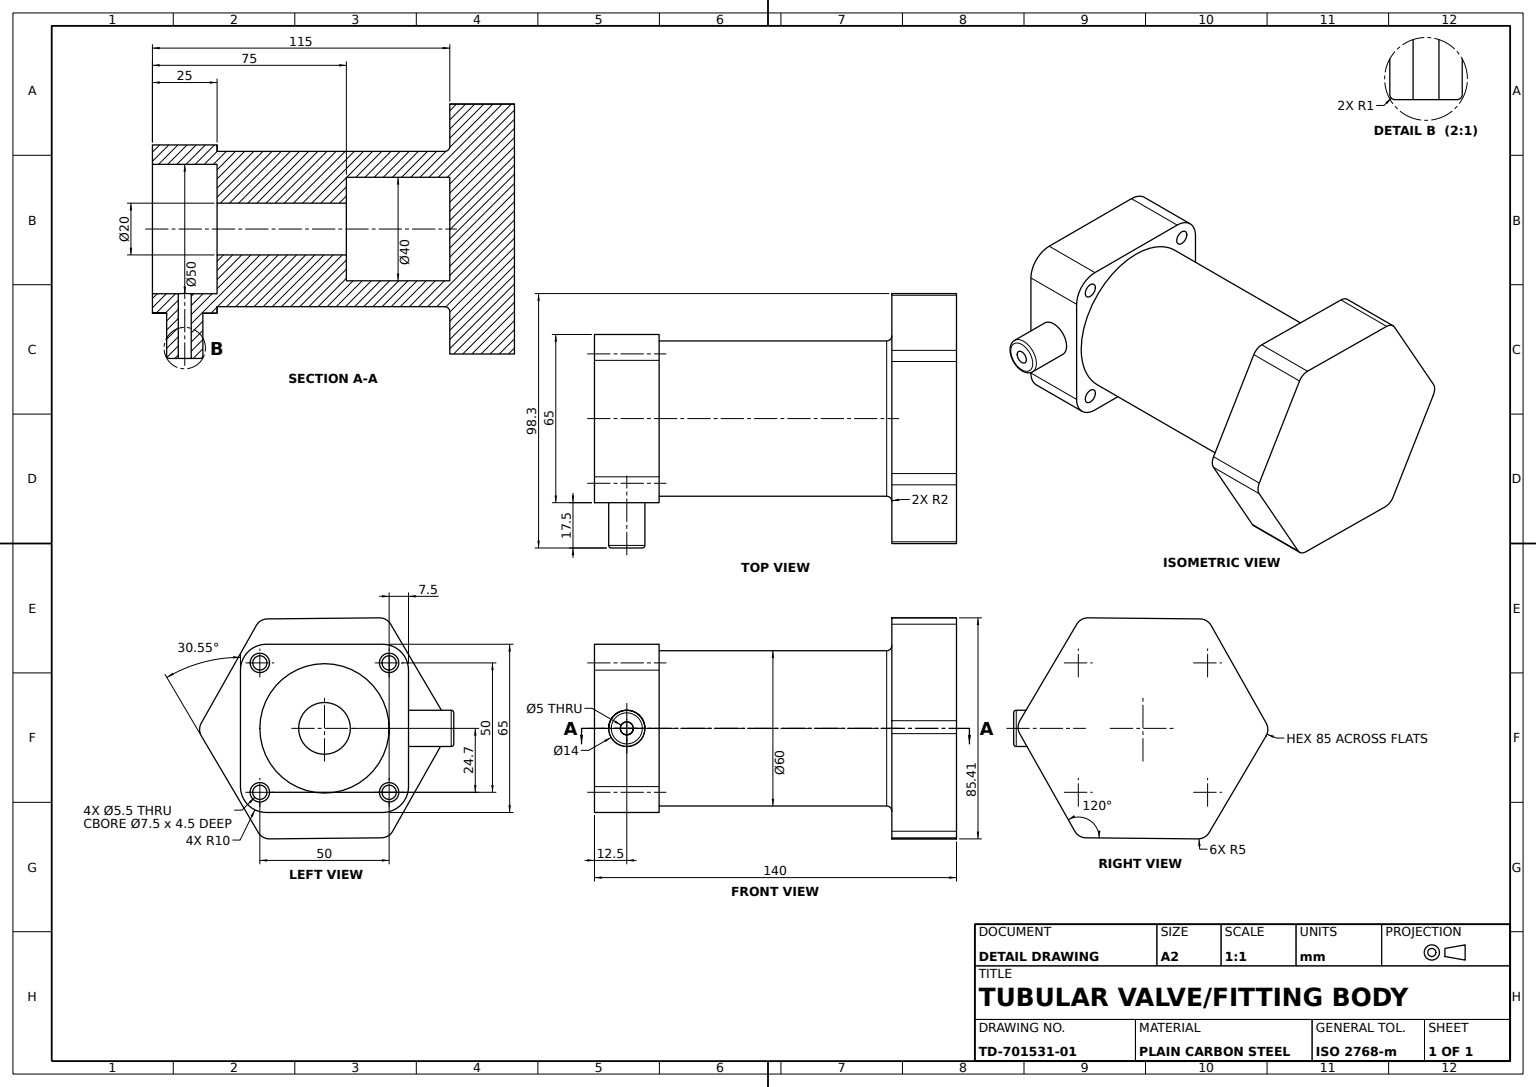
from build123d import *

# Parameters (mm, degrees)
HEX_BODY_DEPTH                     = 25
BODY_PROFILE_60_R                  = 30
BODY_CYLINDER_60_DEPTH             = 90
SQUARE_FLANGE_DEPTH                = 25
FLANGE_BORE_PROFILE_50_R           = 25
FLANGE_BORE_50_DEPTH               = 25
THROUGH_BORE_PROFILE_20_R          = 10
THROUGH_BORE_20_DEPTH              = 50
HEX_END_BORE_PROFILE_40_R          = 20
HEX_END_BORE_40_DEPTH              = 40
HEX_EDGE_FILLET_R5_A_R             = 5
HEX_EDGE_FILLET_R5_B_R             = 5
HEX_EDGE_FILLET_R5_C_R             = 5
HEX_EDGE_FILLET_R5_D_R             = 5
HEX_EDGE_FILLET_R5_E_R             = 5
HEX_EDGE_FILLET_R5_F_R             = 5
COUNTERBORE_PROFILE_4X_7_5_R       = 3.75
MOUNTING_COUNTERBORES_4X_7_5_DEPTH = 4.5
MOUNTING_HOLE_PROFILE_4X_5_5_R     = 2.75
MOUNTING_HOLES_4X_5_5_DEPTH        = 20.5
PORT_BOSS_PROFILE_14_R             = 7
PRESSURE_PORT_BOSS_14_DEPTH        = 17.5
PORT_BOSS_TIP_FILLET_R1_R          = 1
PORT_HOLE_PROFILE_5_R              = 2.5
PORT_HOLE_5_DEPTH                  = 28
BODY_TO_HEX_FILLET_R2_R            = 2


with BuildPart() as part:
    # Hex Profile → Hex Body (new body)
    with BuildSketch(Plane.XY):
        Polygon((24.12843754, 42.733497812), (-24.944075927, 42.262588769), (-49.072513467, -0.470909043), (-24.12843754, -42.733497812), (24.944075927, -42.262588769), (49.072513467, 0.470909043), align=None)
    extrude(amount=HEX_BODY_DEPTH)

    # Body Profile Ø60 → Body Cylinder Ø60 (add)
    with BuildSketch(Plane.XY.offset(25)):
        with Locations(Location((0, 0, 0), (0, 0, 180))):
            Circle(BODY_PROFILE_60_R)
    extrude(amount=BODY_CYLINDER_60_DEPTH)

    # Flange Profile 65x65 → Square Flange (add)
    with BuildSketch(Plane.XY.offset(115)):
        with BuildLine():
            Line((-22.5, -32.5), (22.5, -32.5))
            ThreePointArc((22.5, -32.5), (29.571067812, -29.571067812), (32.5, -22.5))
            Line((32.5, -22.5), (32.5, 22.5))
            ThreePointArc((32.5, 22.5), (29.571067812, 29.571067812), (22.5, 32.5))
            Line((22.5, 32.5), (-22.5, 32.5))
            ThreePointArc((-22.5, 32.5), (-29.571067812, 29.571067812), (-32.5, 22.5))
            Line((-32.5, 22.5), (-32.5, -22.5))
            ThreePointArc((-32.5, -22.5), (-29.571067812, -29.571067812), (-22.5, -32.5))
        make_face()
    extrude(amount=SQUARE_FLANGE_DEPTH)

    # Flange Bore Profile Ø50 → Flange Bore Ø50 (cut)
    with BuildSketch(Plane.XY.offset(140)):
        Circle(FLANGE_BORE_PROFILE_50_R)
    extrude(amount=-FLANGE_BORE_50_DEPTH, mode=Mode.SUBTRACT)

    # Through Bore Profile Ø20 → Through Bore Ø20 (cut)
    with BuildSketch(Plane.XY.offset(115)):
        Circle(THROUGH_BORE_PROFILE_20_R)
    extrude(amount=-THROUGH_BORE_20_DEPTH, mode=Mode.SUBTRACT)

    # Hex End Bore Profile Ø40 → Hex End Bore Ø40 (cut)
    with BuildSketch(Plane.XY.offset(65)):
        Circle(HEX_END_BORE_PROFILE_40_R)
    extrude(amount=-HEX_END_BORE_40_DEPTH, mode=Mode.SUBTRACT)

    # Hex Edge Fillet R5 A
    hex_edge_fillet_r5_a_edges = [part.edges().sort_by_distance(p)[0] for p in [
        (24.12843754, 42.733497812, 12.5),
    ]]
    fillet(hex_edge_fillet_r5_a_edges, radius=HEX_EDGE_FILLET_R5_A_R)

    # Hex Edge Fillet R5 B
    hex_edge_fillet_r5_b_edges = [part.edges().sort_by_distance(p)[0] for p in [
        (49.072513467, 0.470909043, 12.5),
    ]]
    fillet(hex_edge_fillet_r5_b_edges, radius=HEX_EDGE_FILLET_R5_B_R)

    # Hex Edge Fillet R5 C
    hex_edge_fillet_r5_c_edges = [part.edges().sort_by_distance(p)[0] for p in [
        (-24.944075927, 42.262588769, 12.5),
    ]]
    fillet(hex_edge_fillet_r5_c_edges, radius=HEX_EDGE_FILLET_R5_C_R)

    # Hex Edge Fillet R5 D
    hex_edge_fillet_r5_d_edges = [part.edges().sort_by_distance(p)[0] for p in [
        (-49.072513467, -0.470909043, 12.5),
    ]]
    fillet(hex_edge_fillet_r5_d_edges, radius=HEX_EDGE_FILLET_R5_D_R)

    # Hex Edge Fillet R5 E
    hex_edge_fillet_r5_e_edges = [part.edges().sort_by_distance(p)[0] for p in [
        (-24.12843754, -42.733497812, 12.5),
    ]]
    fillet(hex_edge_fillet_r5_e_edges, radius=HEX_EDGE_FILLET_R5_E_R)

    # Hex Edge Fillet R5 F
    hex_edge_fillet_r5_f_edges = [part.edges().sort_by_distance(p)[0] for p in [
        (24.944075927, -42.262588769, 12.5),
    ]]
    fillet(hex_edge_fillet_r5_f_edges, radius=HEX_EDGE_FILLET_R5_F_R)

    # Counterbore Profile 4xØ7.5 → Mounting Counterbores 4xØ7.5 (cut)
    with BuildSketch(Plane.XY.offset(140)):
        with Locations((-25, 25.295084972)):
            Circle(COUNTERBORE_PROFILE_4X_7_5_R)
        with Locations((-25, -24.704915028)):
            Circle(COUNTERBORE_PROFILE_4X_7_5_R)
        with Locations(Location((25, -24.704915028, 0), (0, 0, 180))):
            Circle(COUNTERBORE_PROFILE_4X_7_5_R)
        with Locations(Location((25, 25.295084972, 0), (0, 0, 180))):
            Circle(COUNTERBORE_PROFILE_4X_7_5_R)
    extrude(amount=-MOUNTING_COUNTERBORES_4X_7_5_DEPTH, mode=Mode.SUBTRACT)

    # Mounting Hole Profile 4xØ5.5 → Mounting Holes 4xØ5.5 (cut)
    with BuildSketch(Plane.XY.offset(135.5)):
        with Locations((-25, 25.295084972)):
            Circle(MOUNTING_HOLE_PROFILE_4X_5_5_R)
        with Locations((25, 25.295084972)):
            Circle(MOUNTING_HOLE_PROFILE_4X_5_5_R)
        with Locations((25, -24.704915028)):
            Circle(MOUNTING_HOLE_PROFILE_4X_5_5_R)
        with Locations((-25, -24.704915028)):
            Circle(MOUNTING_HOLE_PROFILE_4X_5_5_R)
    extrude(amount=-MOUNTING_HOLES_4X_5_5_DEPTH, mode=Mode.SUBTRACT)

    # Port Boss Profile Ø14 → Pressure Port Boss Ø14 (add)
    with BuildSketch(Plane(origin=(32.5, 0, 0), x_dir=(0, 0, -1), z_dir=(1, 0, 0))):
        with Locations((-127.5, 0)):
            Circle(PORT_BOSS_PROFILE_14_R)
    extrude(amount=PRESSURE_PORT_BOSS_14_DEPTH)

    # Port Boss Tip Fillet R1
    port_boss_tip_fillet_r1_edges = [part.edges().sort_by_distance(p)[0] for p in [
        (50, 0, 134.5),
    ]]
    fillet(port_boss_tip_fillet_r1_edges, radius=PORT_BOSS_TIP_FILLET_R1_R)

    # Port Hole Profile Ø5 → Port Hole Ø5 (cut)
    with BuildSketch(Plane(origin=(50, 0, 0), x_dir=(0, 0, -1), z_dir=(1, 0, 0))):
        with Locations((-127.5, 0)):
            Circle(PORT_HOLE_PROFILE_5_R)
    extrude(amount=-PORT_HOLE_5_DEPTH, mode=Mode.SUBTRACT)

    # Body to Hex Fillet R2
    body_to_hex_fillet_r2_edges = [part.edges().sort_by_distance(p)[0] for p in [
        (30, 0, 25),
    ]]
    fillet(body_to_hex_fillet_r2_edges, radius=BODY_TO_HEX_FILLET_R2_R)


solid = part.part
